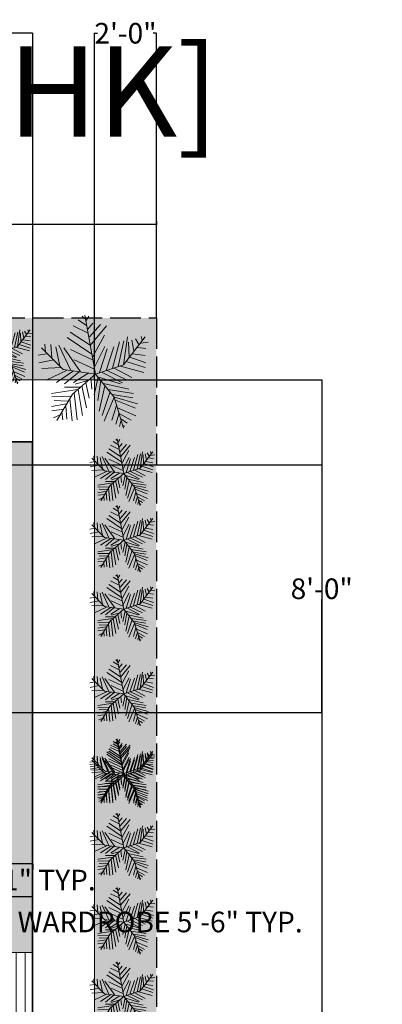
# Model space of a CAD drawing. Units: inches. Extents: x 853 to 1550, y 485 to 1596.
# Tile 18 of 18: x 1409 to 1550, y 1208 to 1590. Entities that reach past the tile are written whole.
import ezdxf

# ---------------------------------------------------------------- set-up
doc = ezdxf.new("R2010")
doc.units = ezdxf.units.IN
doc.header["$MEASUREMENT"] = 0
doc.linetypes.add('ACAD_ISO02W100', pattern=[15, 12, -3])
for name, color, linetype, lineweight in [('A-ANNO-DIMS', 2, 'Continuous', 18), ('A-ANNO-TEXT', 250, 'Continuous', 25), ('A-WALL-PATT', 250, 'Continuous', 13), ('C-PROP', 8, 'ACAD_ISO02W100', 25), ('L-PLNT-TREE', 106, 'Continuous', 13), ('lawn', 106, 'Continuous', 18), ('walls', 250, 'Continuous', 35), ('windows', 4, 'Continuous', 18)]:
    doc.layers.add(name, color=color, linetype=linetype, lineweight=lineweight)
doc.layers.add('L-PLNT-PATT', color=85, linetype='Continuous', lineweight=13, true_color=0x58ba48)
doc.styles.get("Standard").update_dxf_attribs({"font": 'arial.ttf'})
doc.dimstyles.get("Standard").update_dxf_attribs({"dimtxt": 8, "dimasz": 0.18, "dimexe": 0.18, "dimexo": 0.0625, "dimgap": 0.09, "dimtad": 0, "dimtih": 1, "dimtoh": 1, "dimzin": 0, "dimdsep": 46, "dimlunit": 3, "dimtxsty": 'Standard', "dimcen": 0.09, "dimadec": 0, "dimazin": 0, "dimtfac": 1, "dimtofl": 0, "dimtmove": 0, "dimatfit": 3, "dimfxl": 1, "dimtolj": 1, "dimtzin": 0, "dimarcsym": 0})

# ---------------------------------------------------------------- blocks, each defined once
blk = doc.blocks.new('*U18')
for p, q in [((-8.737, 47.138), (-17.069, 52.711)), ((-10.186, 53.64), (-13.084, 55.962)), ((0, 0), (-10.5, 57)), ((-9.099, 51.782), (-6.563, 55.962)), ((-7.65, 43.423), (-2.578, 49.46)), ((-5.839, 35.992), (4.667, 48.067)), ((-5.114, 28.097), (-24.676, 40.636)), ((-7.288, 39.707), (-21.778, 46.673)), ((-5.114, 27.632), (10.463, 46.673)), ((-48.585, 21.131), (-49.309, 29.026)), ((-3.665, 19.273), (-27.574, 35.527)), ((-2.941, 16.486), (8.652, 37.85)), ((16.259, 5.805), (23.142, 31.348)), ((22.055, 7.198), (27.489, 32.277)), ((27, 9), (48, 36)), ((27.127, 9.056), (31.112, 35.992)), ((31.836, 30.883), (32.561, 16.486)), ((35.096, 32.741), (37.27, 22.524)), ((38.719, 34.134), (41.979, 28.561)), ((43.791, 29.954), (51.036, 30.883)), ((44.153, 36.456), (45.239, 32.741)), ((-47.498, 19.737), (-55.83, 18.344)), ((-31.5, 4.5), (-52.5, 25.5)), ((-43.513, 28.561), (-42.427, 15.558)), ((-38.442, 26.239), (-34.819, 7.663)), ((-35.544, 28.097), (-24.314, 3.947)), ((-14.533, 2.09), (-30.834, 25.31)), ((-24.314, 23.917), (-2.941, 13.7)), ((-1.129, 6.734), (9.014, 26.704)), ((3.942, 1.625), (11.187, 24.381)), ((10.101, 3.483), (17.708, 26.239)), ((36.183, 19.737), (48.137, 17.88)), ((40.53, 25.775), (48.862, 24.846)), ((-40.615, 13.7), (-55.105, 10.913)), ((-20.691, 13.7), (-1.129, 4.876)), ((29.662, 12.307), (48.137, 6.269)), ((33.285, 16.486), (48.862, 10.913)), ((-33.37, 6.269), (-52.207, 5.34)), ((-28.299, 3.483), (-47.86, -5.805)), ((-21.416, 3.018), (-38.079, -8.128)), ((0, 0), (-31.5, 4.5)), ((-15.982, 2.09), (-30.11, -9.521)), ((0, 0), (-22.5, -19.5)), ((-6.563, 1.161), (-21.416, -8.128)), ((0, 0), (27, 9)), ((0, 0), (18, -22.5)), ((6.478, 1.625), (26.04, -8.592)), ((11.187, 3.483), (30.749, -5.805)), ((18.07, 5.805), (35.096, -3.483)), ((24.229, 7.663), (46.688, 1.625)), ((-6.563, -5.805), (-19.967, -9.985)), ((-9.461, -8.592), (-6.201, -23.453)), ((-4.752, -3.483), (-3.665, -14.629)), ((2.493, -3.019), (-1.491, -20.202)), ((1.769, -2.555), (24.229, -9.521)), ((5.029, -6.27), (2.131, -25.775)), ((7.565, -9.056), (32.198, -14.629)), ((-17.431, -15.094), (-42.789, -18.809)), ((-15.257, -12.772), (-30.11, -12.772)), ((-20.691, -18.345), (-17.793, -44.352)), ((-17.069, -15.094), (-12.721, -40.172)), ((-13.446, -11.378), (-8.737, -32.741)), ((9.014, -11.378), (3.58, -35.992)), ((14.085, -16.951), (6.478, -40.172)), ((12.274, -15.094), (36.907, -18.809)), ((-24.314, -21.596), (-42.427, -22.06)), ((-26.849, -26.24), (-40.253, -25.775)), ((-22.5, -19.5), (-37.5, -45)), ((-25.038, -23.918), (-22.865, -45.281)), ((18.07, -22.524), (8.289, -45.745)), ((16.259, -19.738), (36.183, -22.989)), ((18, -22.5), (27, -52.5)), ((18.433, -22.524), (40.53, -29.026)), ((19.157, -25.311), (38.719, -33.206)), ((-28.299, -29.026), (-42.789, -31.348)), ((-30.834, -34.135), (-42.427, -35.528)), ((-32.646, -36.921), (-31.921, -44.352)), ((-29.023, -30.884), (-27.936, -43.887)), ((20.244, -30.419), (15.897, -44.816)), ((22.78, -37.85), (19.519, -48.532)), ((21.331, -32.741), (39.081, -40.636)), ((-34.457, -39.708), (-40.978, -42.494)), ((22.78, -38.314), (34.372, -44.816)), ((24.591, -45.745), (23.142, -50.854)), ((24.591, -43.423), (30.749, -47.603)), ((26.764, -49.925), (28.213, -50.854))]:
    blk.add_line(p, q)
blk = doc.blocks.new('*D22')
at = {"layer": 'A-ANNO-DIMS', "color": 0, "lineweight": -2, "transparency": 16777216}
for p, q in [((933.94, 1511.65), (933.94, 1510.09)), ((1461.94, 1511.65), (1461.94, 1510.09)), ((934.12, 1510.27), (1190.9, 1510.27)), ((1461.76, 1510.27), (1204.98, 1510.27))]:
    blk.add_line(p, q, dxfattribs=at)
at = {"layer": 'A-ANNO-DIMS', "color": 0, "transparency": 16777216}
for points in [[(934.12, 1510.3), (934.12, 1510.24), (933.94, 1510.27)], [(1461.76, 1510.3), (1461.76, 1510.24), (1461.94, 1510.27)]]:
    blk.add_solid(points, dxfattribs=at)
at = {"layer": 'Defpoints', "color": 0, "transparency": 16777216}
for p in [(933.94, 1511.71), (1461.94, 1511.71), (1461.94, 1510.27)]:
    blk.add_point(p, dxfattribs=at)
at = {"layer": 'A-ANNO-DIMS', "color": 0, "transparency": 16777216, "insert": (1197.94, 1510.27), "char_height": 8, "attachment_point": 5}
blk.add_mtext("\\A1;40'", dxfattribs=at)
blk = doc.blocks.new('WIN-94IN')
for p, q in [((0, 94.25), (9, 94.25)), ((0, 0), (0, 94.25)), ((2.54, 94.25), (2.54, 0)), ((6.1, 0), (6.1, 94.25)), ((9, 94.25), (9, 0)), ((9, 0), (0, 0)), ((2.54, 0), (6.1, 0))]:
    blk.add_line(p, q)
blk = doc.blocks.new('*D43')
at = {"layer": 'A-ANNO-DIMS', "color": 0, "lineweight": -2, "transparency": 16777216}
for p, q in [((1338.32, 1249.77), (1338.32, 1239.78)), ((1404.11, 1249.77), (1404.11, 1239.78)), ((1338.5, 1239.96), (1403.93, 1239.96)), ((1404.11, 1239.96), (1404.29, 1239.96))]:
    blk.add_line(p, q, dxfattribs=at)
at = {"layer": 'A-ANNO-DIMS', "color": 0, "transparency": 16777216}
for points in [[(1338.5, 1239.99), (1338.5, 1239.93), (1338.32, 1239.96)], [(1403.93, 1239.99), (1403.93, 1239.93), (1404.11, 1239.96)]]:
    blk.add_solid(points, dxfattribs=at)
at = {"layer": 'Defpoints', "color": 0, "transparency": 16777216}
for p in [(1338.32, 1249.83), (1404.11, 1249.83), (1404.11, 1239.96)]:
    blk.add_point(p, dxfattribs=at)
at = {"layer": 'A-ANNO-DIMS', "color": 0, "transparency": 16777216, "insert": (1463.39, 1239.96), "char_height": 8, "attachment_point": 5}
blk.add_mtext('\\A1;WARDROBE 5\'-6" TYP.', dxfattribs=at)
blk = doc.blocks.new('*D44')
at = {"layer": 'A-ANNO-DIMS', "color": 0, "lineweight": -2, "transparency": 16777216}
for p, q in [((1404.17, 1262.63), (1414.16, 1262.63)), ((1413.98, 1262.45), (1413.98, 1260.34)), ((1413.98, 1250.01), (1413.98, 1252.12)), ((1404.17, 1249.83), (1414.16, 1249.83))]:
    blk.add_line(p, q, dxfattribs=at)
at = {"layer": 'A-ANNO-DIMS', "color": 0, "transparency": 16777216}
for points in [[(1413.95, 1262.45), (1414.01, 1262.45), (1413.98, 1262.63)], [(1413.95, 1250.01), (1414.01, 1250.01), (1413.98, 1249.83)]]:
    blk.add_solid(points, dxfattribs=at)
at = {"layer": 'Defpoints', "color": 0, "transparency": 16777216}
for p in [(1404.11, 1262.63), (1413.98, 1262.63), (1404.11, 1249.83)]:
    blk.add_point(p, dxfattribs=at)
at = {"layer": 'A-ANNO-DIMS', "color": 0, "transparency": 16777216, "insert": (1413.98, 1256.23), "char_height": 8, "attachment_point": 5}
blk.add_mtext('\\A1;1\'-1" TYP.', dxfattribs=at)
blk = doc.blocks.new('*D69')
at = {"layer": 'A-ANNO-DIMS', "color": 0, "lineweight": -2, "transparency": 16777216}
for p, q in [((981.94, 1426.19), (981.94, 1584.65)), ((982.12, 1584.47), (1184.11, 1584.47)), ((1413.76, 1584.47), (1211.77, 1584.47)), ((1413.94, 1426.19), (1413.94, 1584.65))]:
    blk.add_line(p, q, dxfattribs=at)
at = {"layer": 'A-ANNO-DIMS', "color": 0, "transparency": 16777216}
for points in [[(982.12, 1584.5), (982.12, 1584.44), (981.94, 1584.47)], [(1413.76, 1584.5), (1413.76, 1584.44), (1413.94, 1584.47)]]:
    blk.add_solid(points, dxfattribs=at)
at = {"layer": 'Defpoints', "color": 0, "transparency": 16777216}
for p in [(1413.94, 1584.47), (981.94, 1426.13), (1413.94, 1426.13)]:
    blk.add_point(p, dxfattribs=at)
at = {"layer": 'A-ANNO-DIMS', "color": 0, "transparency": 16777216, "insert": (1197.94, 1584.47), "char_height": 8, "attachment_point": 5}
blk.add_mtext('\\A1;36\'-0"', dxfattribs=at)
blk = doc.blocks.new('*D73')
at = {"layer": 'A-ANNO-DIMS', "color": 0, "lineweight": -2, "transparency": 16777216}
for p, q in [((1139.5, 1417.13), (1526.24, 1417.13)), ((1526.06, 1416.95), (1526.06, 1373.3)), ((1526.06, 1321.31), (1526.06, 1364.95)), ((1139.5, 1321.13), (1526.24, 1321.13))]:
    blk.add_line(p, q, dxfattribs=at)
at = {"layer": 'A-ANNO-DIMS', "color": 0, "transparency": 16777216}
for points in [[(1526.03, 1416.95), (1526.09, 1416.95), (1526.06, 1417.13)], [(1526.03, 1321.31), (1526.09, 1321.31), (1526.06, 1321.13)]]:
    blk.add_solid(points, dxfattribs=at)
at = {"layer": 'Defpoints', "color": 0, "transparency": 16777216}
for p in [(1139.44, 1417.13), (1139.44, 1321.13), (1526.06, 1321.13)]:
    blk.add_point(p, dxfattribs=at)
at = {"layer": 'A-ANNO-DIMS', "color": 0, "transparency": 16777216, "insert": (1526.06, 1369.13), "char_height": 8, "attachment_point": 5}
blk.add_mtext('\\A1;8\'-0"', dxfattribs=at)
blk = doc.blocks.new('*D79')
at = {"layer": 'A-ANNO-DIMS', "color": 0, "lineweight": -2, "transparency": 16777216}
for p, q in [((1438, 1450.13), (1526.24, 1450.13)), ((1526.06, 1449.95), (1526.06, 1138.61)), ((1526.06, 818.81), (1526.06, 1130.15)), ((1438, 818.63), (1526.24, 818.63))]:
    blk.add_line(p, q, dxfattribs=at)
at = {"layer": 'A-ANNO-DIMS', "color": 0, "transparency": 16777216}
for points in [[(1526.03, 1449.95), (1526.09, 1449.95), (1526.06, 1450.13)], [(1526.03, 818.81), (1526.09, 818.81), (1526.06, 818.63)]]:
    blk.add_solid(points, dxfattribs=at)
at = {"layer": 'Defpoints', "color": 0, "transparency": 16777216}
for p in [(1437.94, 1450.13), (1526.06, 1450.13), (1437.94, 818.63)]:
    blk.add_point(p, dxfattribs=at)
at = {"layer": 'A-ANNO-DIMS', "color": 0, "transparency": 16777216, "insert": (1526.06, 1134.38), "char_height": 8, "attachment_point": 5}
blk.add_mtext('\\A1;52\'-7 1/2"', dxfattribs=at)
blk = doc.blocks.new('*D83')
at = {"layer": 'A-ANNO-DIMS', "color": 0, "lineweight": -2, "transparency": 16777216}
for p, q in [((1437.94, 1450.19), (1437.94, 1584.65)), ((1438.12, 1584.47), (1439.15, 1584.47)), ((1461.76, 1584.47), (1460.73, 1584.47)), ((1461.94, 1474.19), (1461.94, 1584.65))]:
    blk.add_line(p, q, dxfattribs=at)
at = {"layer": 'A-ANNO-DIMS', "color": 0, "transparency": 16777216}
for points in [[(1438.12, 1584.5), (1438.12, 1584.44), (1437.94, 1584.47)], [(1461.76, 1584.5), (1461.76, 1584.44), (1461.94, 1584.47)]]:
    blk.add_solid(points, dxfattribs=at)
at = {"layer": 'Defpoints', "color": 0, "transparency": 16777216}
for p in [(1461.94, 1584.47), (1461.94, 1474.13), (1437.94, 1450.13)]:
    blk.add_point(p, dxfattribs=at)
at = {"layer": 'A-ANNO-DIMS', "color": 0, "transparency": 16777216, "insert": (1449.94, 1584.47), "char_height": 8, "attachment_point": 5}
blk.add_mtext('\\A1;2\'-0"', dxfattribs=at)

msp = doc.modelspace()

# ---------------------------------------------------------------- hatches: boundary and pattern name
at = {"layer": 'A-WALL-PATT'}
h = msp.add_hatch(color=256, dxfattribs=at)
h.dxf.hatch_style = 1
h.paths.add_polyline_path([(1139.437, 988.732), (1134.937, 988.732), (1134.937, 830.473), (1139.437, 830.473)])
h.paths.add_polyline_path([(1413.937, 1052.227), (1404.937, 1052.227), (1404.937, 1036.129), (1308.937, 1036.129), (1308.937, 1045.033), (1304.437, 1045.033), (1304.437, 1030.033), (1308.937, 1030.033), (1308.937, 1031.629), (1404.937, 1031.629), (1404.937, 863.629), (1365.241, 863.629), (1365.241, 854.629), (1413.937, 854.629)])
h.paths.add_polyline_path([(1413.937, 1133.918), (1404.937, 1133.918), (1404.937, 1100.629), (1304.437, 1100.629), (1304.437, 1078.26), (1308.937, 1078.26), (1308.937, 1096.129), (1404.937, 1096.129), (1404.937, 1084.233), (1407.946, 1084.233), (1413.937, 1084.233)])
h.paths.add_polyline_path([(1268.437, 1417.129), (1288.974, 1417.129), (1288.974, 1426.129), (1244.597, 1426.129), (1244.597, 1417.129), (1263.937, 1417.129), (1263.937, 1321.129), (1260.34, 1321.129), (1260.34, 1316.629), (1263.937, 1316.629), (1263.937, 1283.505), (1268.437, 1283.505)])
h.paths.add_polyline_path([(1413.937, 1426.129), (1360.402, 1426.129), (1360.402, 1417.129), (1404.937, 1417.129), (1404.937, 1249.129), (1268.437, 1249.129), (1268.437, 1254.041), (1268.357, 1254.041), (1263.937, 1254.041), (1263.937, 1244.629), (1404.937, 1244.629), (1404.937, 1228.163), (1413.937, 1228.163)])
h.paths.add_polyline_path([(1215.842, 1426.129), (1184.201, 1426.129), (1184.201, 1417.129), (1199.437, 1417.129), (1199.437, 1321.129), (1172.101, 1321.129), (1172.101, 1316.629), (1229.433, 1316.629), (1229.433, 1321.129), (1203.937, 1321.129), (1203.937, 1417.129), (1215.842, 1417.129)])
h.paths.add_polyline_path([(1139.437, 1417.129), (1155.446, 1417.129), (1155.446, 1426.129), (1091.831, 1426.129), (1091.831, 1417.129), (1134.937, 1417.129), (1134.937, 1289.22), (1139.437, 1289.22), (1139.437, 1316.629), (1143.553, 1316.629), (1143.553, 1321.129), (1139.437, 1321.129)])
h.paths.add_polyline_path([(1139.437, 1255.161), (1134.937, 1255.161), (1134.937, 1249.129), (990.937, 1249.129), (990.937, 1417.129), (1020.402, 1417.129), (1020.402, 1426.129), (981.937, 1426.129), (981.937, 1205.535), (984.477, 1205.535), (990.937, 1205.535), (990.937, 1244.629), (1134.937, 1244.629), (1134.937, 1237.775), (1139.437, 1237.775)])
at = {"layer": 'L-PLNT-PATT'}
h = msp.add_hatch(color=256, dxfattribs=at)
h.dxf.hatch_style = 1
h.paths.add_polyline_path([(1461.937, 1474.129), (933.937, 1474.129), (933.937, 730.129), (933.937, 622.891), (941.686, 622.891), (941.686, 604.895), (957.937, 604.895), (957.937, 1450.129), (1437.937, 1450.129), (1437.937, 604.895), (1454.646, 604.895), (1454.646, 622.891), (1461.937, 622.891), (1461.937, 734.988)])

# ---------------------------------------------------------------- linework, layer by layer
at = {"layer": 'C-PROP'}
for p, q in [((933.937, 1474.129), (1461.937, 1474.129)), ((1461.937, 1474.129), (1461.937, 730.129))]:
    msp.add_line(p, q, dxfattribs=at)
at = {"layer": 'lawn'}
for p, q in [((957.937, 1450.129), (1437.937, 1450.129)), ((1437.937, 1450.129), (1437.937, 818.629))]:
    msp.add_line(p, q, dxfattribs=at)
at = {"layer": 'walls'}
for p, q in [((981.937, 1426.129), (1413.937, 1426.129)), ((1413.937, 1426.129), (1413.937, 854.629))]:
    msp.add_line(p, q, dxfattribs=at)

# ---------------------------------------------------------------- block references
at = {"layer": 'L-PLNT-TREE'}
for p, xscale, yscale, zscale in [((1401.667, 1460.956), 0.2357951711934384, 0.2357951711934384, 0.2357951711934384), ((1438.348, 1452.362), 0.3996992985476591, 0.3996992985476591, 0.3996992985476591), ((1449.245, 1413.762), 0.2357951711934384, 0.2357951711934384, 0.2357951711934384), ((1449.245, 1387.934), 0.2357951711934384, 0.2357951711934384, 0.2357951711934384), ((1449.245, 1361.215), 0.2357951711934384, 0.2357951711934384, 0.2357951711934384), ((1449.245, 1328.341), 0.2357951711934384, 0.2357951711934384, 0.2357951711934384), ((1449.245, 1297.533), 0.2357951711934384, 0.2357951711934384, 0.2357951711934384), ((1449.245, 1296.649), 0.2357951711934384, 0.2357951711934384, 0.2357951711934384), ((1449.245, 1268.695), 0.2357951711934384, 0.2357951711934384, 0.2357951711934384), ((1449.245, 1239.907), 0.2357951711934384, 0.2357951711934384, 0.2357951711934384), ((1449.245, 1211.111), 0.2357951711934384, 0.2357951711934384, 0.2357951711934384)]:
    msp.add_blockref('*U18', p, dxfattribs=dict(at, xscale=xscale, yscale=yscale, zscale=zscale))
at = {"layer": 'windows'}
msp.add_blockref('WIN-94IN', (1404.937, 1133.918), dxfattribs=at)

# ---------------------------------------------------------------- texts
at = {"layer": 'A-ANNO-TEXT'}
msp.add_text('40X60 HOUSE PLAN [4BHK]', height=35.05469, dxfattribs=at).set_placement((883.136, 1544.353))

# ---------------------------------------------------------------- dimensions: what is measured, and where the dimension line sits
at = {"layer": 'A-ANNO-DIMS'}
for base, p1, p2, picture, middle in [((1413.937, 1584.468), (981.937, 1426.129), (1413.937, 1426.129), '*D69', (1197.937, 1584.468)), ((1461.937, 1584.468), (1437.937, 1450.129), (1461.937, 1474.129), '*D83', (1449.937, 1584.468))]:
    dim = msp.add_linear_dim(base=base, p1=p1, p2=p2, dimstyle='Standard', override={"dimdec": 1, "dimlfac": 1, "dimrnd": 0, "dimzin": 1, "dimdsep": 46, "dimlunit": 4, "dimfrac": 2}, dxfattribs=at)
    dim.commit()
    dim.dimension.update_dxf_attribs({"geometry": picture, "text_midpoint": middle})
for base, p1, p2, text, override, picture, middle in [((1461.937, 1510.271), (933.937, 1511.712), (1461.937, 1511.712), "40'", {"dimclrd": 0, "dimclre": 0, "dimclrt": 0}, '*D22', (1197.937, 1510.271)), ((1404.112, 1239.964), (1338.324, 1249.832), (1404.112, 1249.832), 'WARDROBE <> TYP.', {"dimdec": 1, "dimlfac": 1, "dimrnd": 0, "dimzin": 1, "dimdsep": 46, "dimlunit": 4, "dimfrac": 2}, '*D43', (1463.389, 1239.964))]:
    dim = msp.add_linear_dim(base=base, p1=p1, p2=p2, text=text, dimstyle='Standard', override=override, dxfattribs=at)
    dim.commit()
    dim.dimension.update_dxf_attribs({"geometry": picture, "text_midpoint": middle})
for base, p1, p2, picture, middle in [((1526.064, 1450.129), (1437.937, 818.629), (1437.937, 1450.129), '*D79', (1526.064, 1134.379)), ((1526.064, 1321.129), (1139.437, 1417.129), (1139.437, 1321.129), '*D73', (1526.064, 1369.129))]:
    dim = msp.add_linear_dim(base=base, p1=p1, p2=p2, angle=90, dimstyle='Standard', override={"dimdec": 1, "dimlfac": 1, "dimrnd": 0, "dimzin": 1, "dimdsep": 46, "dimlunit": 4, "dimfrac": 2}, dxfattribs=at)
    dim.commit()
    dim.dimension.update_dxf_attribs({"geometry": picture, "text_midpoint": middle})
dim = msp.add_linear_dim(base=(1413.98, 1262.63), p1=(1404.112, 1249.832), p2=(1404.112, 1262.63), angle=90, text='<> TYP.', dimstyle='Standard', override={"dimdec": 1, "dimlfac": 1, "dimrnd": 0, "dimzin": 1, "dimdsep": 46, "dimlunit": 4, "dimfrac": 2}, dxfattribs=at)
dim.commit()
dim.dimension.update_dxf_attribs({"geometry": '*D44', "text_midpoint": (1413.98, 1256.231)})

doc.saveas('drawing.dxf')
